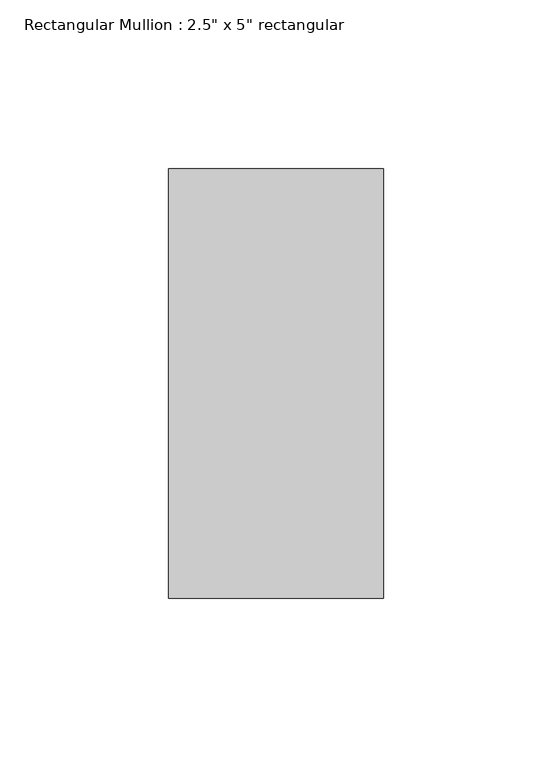
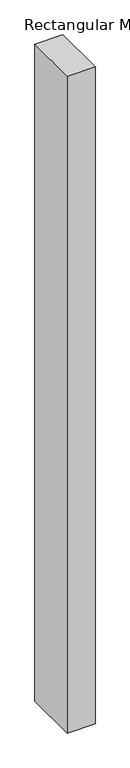
"""IFC4 building model written with IfcOpenShell, lengths in millimetres: member geometry."""

from ifc_helpers import new_model, si_unit, frame, origin, place, context, project, spatial, polyline, outline, extrude, source, transform, mapped, element, save


def member_3042558b(model_context):
    return source(origin(), model_context, "Body", "SweptSolid", [
        extrude(outline(polyline([(0.0, 63.5), (0.0, -63.5), (-63.5, -63.5), (-63.5, 63.5), (0.0, 63.5)])), frame((0.0, 0.0, -1580.0534505), z_axis=(0.0, 0.0, 1.0), x_axis=(1.0, 0.0, 0.0)), (0.0, 0.0, 1.0), 1580.0534505),
    ])


if __name__ == "__main__":
    model = new_model("IFC4")
    model_context = context("Model", 3, world=origin())
    ifc_project = project(units=[si_unit("LENGTHUNIT", "METRE", prefix="MILLI")], contexts=[model_context])
    site = spatial("IfcSite", under=ifc_project)
    building = spatial("IfcBuilding", under=site)
    placement = place(None, origin())
    member_shape = member_3042558b(model_context)
    element("IfcMember", 1, ObjectType="Rectangular Mullion : 2.5\" x 5\" rectangular", at=placement, inside=building, context=model_context, shape_type="MappedRepresentation", body=[
        mapped(member_shape, transform((0.0, 0.0, 0.0), x_axis=(1.0, 0.0, 0.0), y_axis=(0.0, 1.0, 0.0), z_axis=(0.0, 0.0, 1.0))),
    ])
    save(model, "model.ifc")

# Revit data of these elements
# Type "Rectangular Mullion : 2.5\" x 5\" rectangular"
#   built-in parameter 1007304 = 0.416667 (stored number, unit not read)
#   built-in parameter 1007301 = 0.104167 (stored number, unit not read)
#   built-in parameter 1007300 = 0.104167 (stored number, unit not read)
# Element 1 (IfcMember, "Rectangular Mullion : 2.5\" x 5\" rectangular")
#   Materials on its faces: "Aluminum"
# Materials
#   "Aluminum": class "Metal", colour RGB 247 247 247, transparency 0, Description = "Aluminum 6061", Cost = 0
